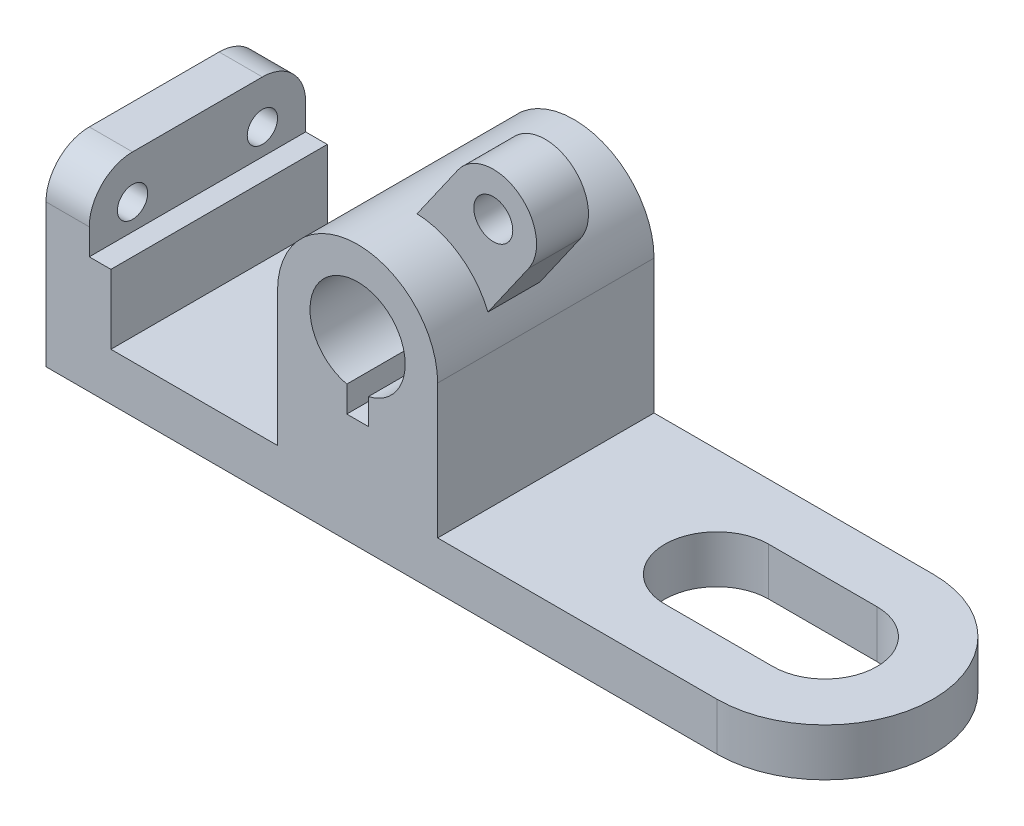
ISO-10303-21;
HEADER;
FILE_DESCRIPTION(('STEP AP214'),'2;1');
FILE_NAME('part.step','',(''),(''),'','','');
FILE_SCHEMA(('AUTOMOTIVE_DESIGN { 1 0 10303 214 1 1 1 1 }'));
ENDSEC;
DATA;
#1=APPLICATION_CONTEXT('core data for automotive mechanical design processes');
#2=APPLICATION_PROTOCOL_DEFINITION('international standard','automotive_design',2000,#1);
#3=PRODUCT_CONTEXT('',#1,'mechanical');
#4=PRODUCT('Part','Part','',(#3));
#5=PRODUCT_RELATED_PRODUCT_CATEGORY('part','',(#4));
#6=PRODUCT_DEFINITION_FORMATION('','',#4);
#7=PRODUCT_DEFINITION_CONTEXT('part definition',#1,'design');
#8=PRODUCT_DEFINITION('design','',#6,#7);
#9=PRODUCT_DEFINITION_SHAPE('','',#8);
#10=(LENGTH_UNIT() NAMED_UNIT(*) SI_UNIT(.MILLI.,.METRE.));
#11=(NAMED_UNIT(*) PLANE_ANGLE_UNIT() SI_UNIT($,.RADIAN.));
#12=(NAMED_UNIT(*) SI_UNIT($,.STERADIAN.) SOLID_ANGLE_UNIT());
#13=UNCERTAINTY_MEASURE_WITH_UNIT(LENGTH_MEASURE(1.E-05),#10,'distance_accuracy_value','');
#14=(GEOMETRIC_REPRESENTATION_CONTEXT(3) GLOBAL_UNCERTAINTY_ASSIGNED_CONTEXT((#13)) GLOBAL_UNIT_ASSIGNED_CONTEXT((#10,
#11,#12)) REPRESENTATION_CONTEXT('',''));
#15=CARTESIAN_POINT('',(0.,0.,0.));
#16=DIRECTION('',(0.,0.,1.));
#17=DIRECTION('',(1.,0.,0.));
#18=AXIS2_PLACEMENT_3D('',#15,#16,#17);
#19=CARTESIAN_POINT('',(-83.,42.,-25.));
#20=DIRECTION('',(0.,0.,1.));
#21=DIRECTION('',(1.,0.,0.));
#22=AXIS2_PLACEMENT_3D('',#19,#20,#21);
#23=CYLINDRICAL_SURFACE('',#22,18.5);
#24=CARTESIAN_POINT('',(-83.,42.,25.));
#25=DIRECTION('',(0.,0.,1.));
#26=DIRECTION('',(1.,0.,0.));
#27=AXIS2_PLACEMENT_3D('',#24,#25,#26);
#28=CIRCLE('',#27,18.5);
#29=CARTESIAN_POINT('',(-64.5,42.,25.));
#30=VERTEX_POINT('',#29);
#31=CARTESIAN_POINT('',(-101.5,42.,25.));
#32=VERTEX_POINT('',#31);
#33=EDGE_CURVE('E272',#30,#32,#28,.T.);
#34=ORIENTED_EDGE('',*,*,#33,.F.);
#35=DIRECTION('',(0.,0.,1.));
#36=VECTOR('',#35,1.);
#37=CARTESIAN_POINT('',(-64.5,42.,-25.));
#38=LINE('',#37,#36);
#39=CARTESIAN_POINT('',(-64.5,42.,-25.));
#40=VERTEX_POINT('',#39);
#41=EDGE_CURVE('E303',#40,#30,#38,.T.);
#42=ORIENTED_EDGE('',*,*,#41,.F.);
#43=CARTESIAN_POINT('',(-83.,42.,-25.));
#44=DIRECTION('',(0.,0.,1.));
#45=DIRECTION('',(1.,0.,0.));
#46=AXIS2_PLACEMENT_3D('',#43,#44,#45);
#47=CIRCLE('',#46,18.5);
#48=CARTESIAN_POINT('',(-101.5,42.,-25.));
#49=VERTEX_POINT('',#48);
#50=EDGE_CURVE('E255',#40,#49,#47,.T.);
#51=ORIENTED_EDGE('',*,*,#50,.T.);
#52=DIRECTION('',(0.,0.,1.));
#53=VECTOR('',#52,1.);
#54=CARTESIAN_POINT('',(-101.5,42.,-25.));
#55=LINE('',#54,#53);
#56=EDGE_CURVE('E301',#49,#32,#55,.T.);
#57=ORIENTED_EDGE('',*,*,#56,.T.);
#58=EDGE_LOOP('',(#34,#42,#51,#57));
#59=FACE_BOUND('',#58,.T.);
#60=CARTESIAN_POINT('',(-83.,42.,12.));
#61=DIRECTION('',(0.,0.,-1.));
#62=DIRECTION('',(1.,0.,0.));
#63=AXIS2_PLACEMENT_3D('',#60,#61,#62);
#64=CIRCLE('',#63,18.5);
#65=CARTESIAN_POINT('',(-82.264157442559,60.4853600378964,12.));
#66=VERTEX_POINT('',#65);
#67=CARTESIAN_POINT('',(-65.8811165567791,49.0138313108756,12.));
#68=VERTEX_POINT('',#67);
#69=EDGE_CURVE('E227',#66,#68,#64,.T.);
#70=ORIENTED_EDGE('',*,*,#69,.F.);
#71=DIRECTION('',(0.,0.,-1.));
#72=VECTOR('',#71,1.);
#73=CARTESIAN_POINT('',(-82.264157442559,60.4853600378964,12.));
#74=LINE('',#73,#72);
#75=CARTESIAN_POINT('',(-82.264157442559,60.4853600378964,0.));
#76=VERTEX_POINT('',#75);
#77=EDGE_CURVE('E224',#66,#76,#74,.T.);
#78=ORIENTED_EDGE('',*,*,#77,.T.);
#79=CARTESIAN_POINT('',(-83.,42.,0.));
#80=DIRECTION('',(0.,0.,-1.));
#81=DIRECTION('',(1.,0.,0.));
#82=AXIS2_PLACEMENT_3D('',#79,#80,#81);
#83=CIRCLE('',#82,18.5);
#84=CARTESIAN_POINT('',(-65.8811165567791,49.0138313108756,0.));
#85=VERTEX_POINT('',#84);
#86=EDGE_CURVE('E429',#76,#85,#83,.T.);
#87=ORIENTED_EDGE('',*,*,#86,.T.);
#88=DIRECTION('',(0.,0.,-1.));
#89=VECTOR('',#88,1.);
#90=CARTESIAN_POINT('',(-65.8811165567791,49.0138313108756,12.));
#91=LINE('',#90,#89);
#92=EDGE_CURVE('E246',#68,#85,#91,.T.);
#93=ORIENTED_EDGE('',*,*,#92,.F.);
#94=EDGE_LOOP('',(#70,#78,#87,#93));
#95=FACE_BOUND('',#94,.T.);
#96=ADVANCED_FACE('F41',(#59,#95),#23,.T.);
#97=CARTESIAN_POINT('',(0.,11.,0.));
#98=DIRECTION('',(0.,1.,0.));
#99=DIRECTION('',(0.,0.,1.));
#100=AXIS2_PLACEMENT_3D('',#97,#98,#99);
#101=PLANE('',#100);
#102=DIRECTION('',(-1.,0.,0.));
#103=VECTOR('',#102,1.);
#104=CARTESIAN_POINT('',(0.,11.,-12.));
#105=LINE('',#104,#103);
#106=CARTESIAN_POINT('',(0.,11.,-12.));
#107=VERTEX_POINT('',#106);
#108=CARTESIAN_POINT('',(-25.,11.,-12.));
#109=VERTEX_POINT('',#108);
#110=EDGE_CURVE('E332',#107,#109,#105,.T.);
#111=ORIENTED_EDGE('',*,*,#110,.F.);
#112=CARTESIAN_POINT('',(0.,11.,0.));
#113=DIRECTION('',(0.,1.,0.));
#114=DIRECTION('',(0.,0.,1.));
#115=AXIS2_PLACEMENT_3D('',#112,#113,#114);
#116=CIRCLE('',#115,12.);
#117=CARTESIAN_POINT('',(0.,11.,12.));
#118=VERTEX_POINT('',#117);
#119=EDGE_CURVE('E328',#118,#107,#116,.T.);
#120=ORIENTED_EDGE('',*,*,#119,.F.);
#121=DIRECTION('',(1.,0.,0.));
#122=VECTOR('',#121,1.);
#123=CARTESIAN_POINT('',(0.,11.,12.));
#124=LINE('',#123,#122);
#125=CARTESIAN_POINT('',(-25.,11.,12.));
#126=VERTEX_POINT('',#125);
#127=EDGE_CURVE('E340',#126,#118,#124,.T.);
#128=ORIENTED_EDGE('',*,*,#127,.F.);
#129=CARTESIAN_POINT('',(-25.,11.,0.));
#130=DIRECTION('',(0.,1.,0.));
#131=DIRECTION('',(0.,0.,1.));
#132=AXIS2_PLACEMENT_3D('',#129,#130,#131);
#133=CIRCLE('',#132,12.);
#134=EDGE_CURVE('E331',#109,#126,#133,.T.);
#135=ORIENTED_EDGE('',*,*,#134,.F.);
#136=EDGE_LOOP('',(#111,#120,#128,#135));
#137=FACE_BOUND('',#136,.T.);
#138=DIRECTION('',(-1.,0.,0.));
#139=VECTOR('',#138,1.);
#140=CARTESIAN_POINT('',(0.,11.,-25.));
#141=LINE('',#140,#139);
#142=CARTESIAN_POINT('',(0.,11.,-25.));
#143=VERTEX_POINT('',#142);
#144=CARTESIAN_POINT('',(-64.5,11.,-25.));
#145=VERTEX_POINT('',#144);
#146=EDGE_CURVE('E362',#143,#145,#141,.T.);
#147=ORIENTED_EDGE('',*,*,#146,.T.);
#148=DIRECTION('',(0.,0.,1.));
#149=VECTOR('',#148,1.);
#150=CARTESIAN_POINT('',(-64.5,11.,-25.));
#151=LINE('',#150,#149);
#152=CARTESIAN_POINT('',(-64.5,11.,25.));
#153=VERTEX_POINT('',#152);
#154=EDGE_CURVE('E269',#145,#153,#151,.T.);
#155=ORIENTED_EDGE('',*,*,#154,.T.);
#156=DIRECTION('',(1.,0.,0.));
#157=VECTOR('',#156,1.);
#158=CARTESIAN_POINT('',(0.,11.,25.));
#159=LINE('',#158,#157);
#160=CARTESIAN_POINT('',(0.,11.,25.));
#161=VERTEX_POINT('',#160);
#162=EDGE_CURVE('E368',#153,#161,#159,.T.);
#163=ORIENTED_EDGE('',*,*,#162,.T.);
#164=CARTESIAN_POINT('',(0.,11.,0.));
#165=DIRECTION('',(0.,1.,0.));
#166=DIRECTION('',(0.,0.,1.));
#167=AXIS2_PLACEMENT_3D('',#164,#165,#166);
#168=CIRCLE('',#167,25.);
#169=EDGE_CURVE('E359',#161,#143,#168,.T.);
#170=ORIENTED_EDGE('',*,*,#169,.T.);
#171=EDGE_LOOP('',(#147,#155,#163,#170));
#172=FACE_BOUND('',#171,.T.);
#173=ADVANCED_FACE('F442',(#137,#172),#101,.T.);
#174=DIRECTION('',(0.,0.,1.));
#175=VECTOR('',#174,1.);
#176=CARTESIAN_POINT('',(-101.5,11.,-25.));
#177=LINE('',#176,#175);
#178=CARTESIAN_POINT('',(-101.5,11.,-25.));
#179=VERTEX_POINT('',#178);
#180=CARTESIAN_POINT('',(-101.5,11.,25.));
#181=VERTEX_POINT('',#180);
#182=EDGE_CURVE('E299',#179,#181,#177,.T.);
#183=ORIENTED_EDGE('',*,*,#182,.F.);
#184=CARTESIAN_POINT('',(-140.,11.,-25.));
#185=VERTEX_POINT('',#184);
#186=EDGE_CURVE('E361',#179,#185,#141,.T.);
#187=ORIENTED_EDGE('',*,*,#186,.T.);
#188=DIRECTION('',(0.,0.,1.));
#189=VECTOR('',#188,1.);
#190=CARTESIAN_POINT('',(-140.,11.,-25.));
#191=LINE('',#190,#189);
#192=CARTESIAN_POINT('',(-140.,11.,25.));
#193=VERTEX_POINT('',#192);
#194=EDGE_CURVE('E275',#185,#193,#191,.T.);
#195=ORIENTED_EDGE('',*,*,#194,.T.);
#196=EDGE_CURVE('E369',#193,#181,#159,.T.);
#197=ORIENTED_EDGE('',*,*,#196,.T.);
#198=EDGE_LOOP('',(#183,#187,#195,#197));
#199=FACE_BOUND('',#198,.T.);
#200=ADVANCED_FACE('F452',(#199),#101,.T.);
#201=CARTESIAN_POINT('',(0.,0.,0.));
#202=DIRECTION('',(0.,1.,0.));
#203=DIRECTION('',(0.,0.,1.));
#204=AXIS2_PLACEMENT_3D('',#201,#202,#203);
#205=PLANE('',#204);
#206=CARTESIAN_POINT('',(0.,0.,0.));
#207=DIRECTION('',(0.,1.,0.));
#208=DIRECTION('',(0.,0.,1.));
#209=AXIS2_PLACEMENT_3D('',#206,#207,#208);
#210=CIRCLE('',#209,25.);
#211=CARTESIAN_POINT('',(0.,0.,25.));
#212=VERTEX_POINT('',#211);
#213=CARTESIAN_POINT('',(0.,0.,-25.));
#214=VERTEX_POINT('',#213);
#215=EDGE_CURVE('E360',#212,#214,#210,.T.);
#216=ORIENTED_EDGE('',*,*,#215,.F.);
#217=DIRECTION('',(1.,0.,0.));
#218=VECTOR('',#217,1.);
#219=CARTESIAN_POINT('',(0.,0.,25.));
#220=LINE('',#219,#218);
#221=CARTESIAN_POINT('',(-155.,0.,25.));
#222=VERTEX_POINT('',#221);
#223=EDGE_CURVE('E364',#222,#212,#220,.T.);
#224=ORIENTED_EDGE('',*,*,#223,.F.);
#225=DIRECTION('',(0.,0.,1.));
#226=VECTOR('',#225,1.);
#227=CARTESIAN_POINT('',(-155.,0.,25.));
#228=LINE('',#227,#226);
#229=CARTESIAN_POINT('',(-155.,0.,-25.));
#230=VERTEX_POINT('',#229);
#231=EDGE_CURVE('E376',#230,#222,#228,.T.);
#232=ORIENTED_EDGE('',*,*,#231,.F.);
#233=DIRECTION('',(-1.,0.,0.));
#234=VECTOR('',#233,1.);
#235=CARTESIAN_POINT('',(0.,0.,-25.));
#236=LINE('',#235,#234);
#237=EDGE_CURVE('E373',#214,#230,#236,.T.);
#238=ORIENTED_EDGE('',*,*,#237,.F.);
#239=EDGE_LOOP('',(#216,#224,#232,#238));
#240=FACE_BOUND('',#239,.T.);
#241=CARTESIAN_POINT('',(0.,0.,0.));
#242=DIRECTION('',(0.,1.,0.));
#243=DIRECTION('',(0.,0.,1.));
#244=AXIS2_PLACEMENT_3D('',#241,#242,#243);
#245=CIRCLE('',#244,12.);
#246=CARTESIAN_POINT('',(0.,0.,12.));
#247=VERTEX_POINT('',#246);
#248=CARTESIAN_POINT('',(0.,0.,-12.));
#249=VERTEX_POINT('',#248);
#250=EDGE_CURVE('E293',#247,#249,#245,.T.);
#251=ORIENTED_EDGE('',*,*,#250,.T.);
#252=DIRECTION('',(-1.,0.,0.));
#253=VECTOR('',#252,1.);
#254=CARTESIAN_POINT('',(0.,0.,-12.));
#255=LINE('',#254,#253);
#256=CARTESIAN_POINT('',(-25.,0.,-12.));
#257=VERTEX_POINT('',#256);
#258=EDGE_CURVE('E345',#249,#257,#255,.T.);
#259=ORIENTED_EDGE('',*,*,#258,.T.);
#260=CARTESIAN_POINT('',(-25.,0.,0.));
#261=DIRECTION('',(0.,1.,0.));
#262=DIRECTION('',(0.,0.,1.));
#263=AXIS2_PLACEMENT_3D('',#260,#261,#262);
#264=CIRCLE('',#263,12.);
#265=CARTESIAN_POINT('',(-25.,0.,12.));
#266=VERTEX_POINT('',#265);
#267=EDGE_CURVE('E343',#257,#266,#264,.T.);
#268=ORIENTED_EDGE('',*,*,#267,.T.);
#269=DIRECTION('',(1.,0.,0.));
#270=VECTOR('',#269,1.);
#271=CARTESIAN_POINT('',(0.,0.,12.));
#272=LINE('',#271,#270);
#273=EDGE_CURVE('E335',#266,#247,#272,.T.);
#274=ORIENTED_EDGE('',*,*,#273,.T.);
#275=EDGE_LOOP('',(#251,#259,#268,#274));
#276=FACE_BOUND('',#275,.T.);
#277=ADVANCED_FACE('F498',(#240,#276),#205,.F.);
#278=CARTESIAN_POINT('',(0.,11.,0.));
#279=DIRECTION('',(0.,-1.,0.));
#280=DIRECTION('',(0.,0.,-1.));
#281=AXIS2_PLACEMENT_3D('',#278,#279,#280);
#282=CYLINDRICAL_SURFACE('',#281,25.);
#283=ORIENTED_EDGE('',*,*,#215,.T.);
#284=DIRECTION('',(0.,-1.,0.));
#285=VECTOR('',#284,1.);
#286=CARTESIAN_POINT('',(0.,11.,-25.));
#287=LINE('',#286,#285);
#288=EDGE_CURVE('E390',#143,#214,#287,.T.);
#289=ORIENTED_EDGE('',*,*,#288,.F.);
#290=ORIENTED_EDGE('',*,*,#169,.F.);
#291=DIRECTION('',(0.,-1.,0.));
#292=VECTOR('',#291,1.);
#293=CARTESIAN_POINT('',(0.,11.,25.));
#294=LINE('',#293,#292);
#295=EDGE_CURVE('E379',#161,#212,#294,.T.);
#296=ORIENTED_EDGE('',*,*,#295,.T.);
#297=EDGE_LOOP('',(#283,#289,#290,#296));
#298=FACE_BOUND('',#297,.T.);
#299=ADVANCED_FACE('F501',(#298),#282,.T.);
#300=CARTESIAN_POINT('',(0.,11.,-25.));
#301=DIRECTION('',(0.,0.,1.));
#302=DIRECTION('',(1.,0.,0.));
#303=AXIS2_PLACEMENT_3D('',#300,#301,#302);
#304=PLANE('',#303);
#305=DIRECTION('',(0.,-1.,0.));
#306=VECTOR('',#305,1.);
#307=CARTESIAN_POINT('',(-155.,11.,-25.));
#308=LINE('',#307,#306);
#309=CARTESIAN_POINT('',(-155.,33.,-25.));
#310=VERTEX_POINT('',#309);
#311=EDGE_CURVE('E383',#310,#230,#308,.T.);
#312=ORIENTED_EDGE('',*,*,#311,.F.);
#313=DIRECTION('',(1.,0.,0.));
#314=VECTOR('',#313,1.);
#315=CARTESIAN_POINT('',(0.,33.,-25.));
#316=LINE('',#315,#314);
#317=CARTESIAN_POINT('',(-145.,33.,-25.));
#318=VERTEX_POINT('',#317);
#319=EDGE_CURVE('E388',#310,#318,#316,.T.);
#320=ORIENTED_EDGE('',*,*,#319,.T.);
#321=DIRECTION('',(0.,-1.,0.));
#322=VECTOR('',#321,1.);
#323=CARTESIAN_POINT('',(-145.,-2.51534904016637E-13,-25.));
#324=LINE('',#323,#322);
#325=CARTESIAN_POINT('',(-145.,27.,-25.));
#326=VERTEX_POINT('',#325);
#327=EDGE_CURVE('E315',#318,#326,#324,.T.);
#328=ORIENTED_EDGE('',*,*,#327,.T.);
#329=DIRECTION('',(1.,0.,0.));
#330=VECTOR('',#329,1.);
#331=CARTESIAN_POINT('',(0.,27.,-25.));
#332=LINE('',#331,#330);
#333=CARTESIAN_POINT('',(-140.,27.,-25.));
#334=VERTEX_POINT('',#333);
#335=EDGE_CURVE('E307',#326,#334,#332,.T.);
#336=ORIENTED_EDGE('',*,*,#335,.T.);
#337=DIRECTION('',(0.,-1.,0.));
#338=VECTOR('',#337,1.);
#339=CARTESIAN_POINT('',(-140.,0.,-25.));
#340=LINE('',#339,#338);
#341=EDGE_CURVE('E310',#334,#185,#340,.T.);
#342=ORIENTED_EDGE('',*,*,#341,.T.);
#343=ORIENTED_EDGE('',*,*,#186,.F.);
#344=DIRECTION('',(0.,-1.,0.));
#345=VECTOR('',#344,1.);
#346=CARTESIAN_POINT('',(-101.5,0.,-25.));
#347=LINE('',#346,#345);
#348=EDGE_CURVE('E257',#49,#179,#347,.T.);
#349=ORIENTED_EDGE('',*,*,#348,.F.);
#350=ORIENTED_EDGE('',*,*,#50,.F.);
#351=DIRECTION('',(0.,-1.,0.));
#352=VECTOR('',#351,1.);
#353=CARTESIAN_POINT('',(-64.5,0.,-25.));
#354=LINE('',#353,#352);
#355=EDGE_CURVE('E249',#40,#145,#354,.T.);
#356=ORIENTED_EDGE('',*,*,#355,.T.);
#357=ORIENTED_EDGE('',*,*,#146,.F.);
#358=ORIENTED_EDGE('',*,*,#288,.T.);
#359=ORIENTED_EDGE('',*,*,#237,.T.);
#360=EDGE_LOOP('',(#312,#320,#328,#336,#342,#343,#349,#350,#356,#357,#358,#359));
#361=FACE_BOUND('',#360,.T.);
#362=DIRECTION('',(0.,1.,0.));
#363=VECTOR('',#362,1.);
#364=CARTESIAN_POINT('',(-80.5,0.,-25.));
#365=LINE('',#364,#363);
#366=CARTESIAN_POINT('',(-80.5,25.2878573571857,-25.));
#367=VERTEX_POINT('',#366);
#368=CARTESIAN_POINT('',(-80.5,31.2878573571857,-25.));
#369=VERTEX_POINT('',#368);
#370=EDGE_CURVE('E259',#367,#369,#365,.T.);
#371=ORIENTED_EDGE('',*,*,#370,.T.);
#372=CARTESIAN_POINT('',(-83.,42.,-25.));
#373=DIRECTION('',(0.,0.,1.));
#374=DIRECTION('',(1.,0.,0.));
#375=AXIS2_PLACEMENT_3D('',#372,#373,#374);
#376=CIRCLE('',#375,11.);
#377=CARTESIAN_POINT('',(-85.5,31.2878573571857,-25.));
#378=VERTEX_POINT('',#377);
#379=EDGE_CURVE('E267',#369,#378,#376,.T.);
#380=ORIENTED_EDGE('',*,*,#379,.T.);
#381=DIRECTION('',(0.,1.,0.));
#382=VECTOR('',#381,1.);
#383=CARTESIAN_POINT('',(-85.5,0.,-25.));
#384=LINE('',#383,#382);
#385=CARTESIAN_POINT('',(-85.5,25.2878573571857,-25.));
#386=VERTEX_POINT('',#385);
#387=EDGE_CURVE('E262',#386,#378,#384,.T.);
#388=ORIENTED_EDGE('',*,*,#387,.F.);
#389=DIRECTION('',(1.,0.,0.));
#390=VECTOR('',#389,1.);
#391=CARTESIAN_POINT('',(0.,25.2878573571857,-25.));
#392=LINE('',#391,#390);
#393=EDGE_CURVE('E261',#386,#367,#392,.T.);
#394=ORIENTED_EDGE('',*,*,#393,.T.);
#395=EDGE_LOOP('',(#371,#380,#388,#394));
#396=FACE_BOUND('',#395,.T.);
#397=ADVANCED_FACE('F507',(#361,#396),#304,.F.);
#398=CARTESIAN_POINT('',(-155.,11.,25.));
#399=DIRECTION('',(1.,0.,0.));
#400=DIRECTION('',(0.,0.,-1.));
#401=AXIS2_PLACEMENT_3D('',#398,#399,#400);
#402=PLANE('',#401);
#403=CARTESIAN_POINT('',(-155.,33.,15.));
#404=DIRECTION('',(-1.,0.,0.));
#405=DIRECTION('',(0.,0.,1.));
#406=AXIS2_PLACEMENT_3D('',#403,#404,#405);
#407=CIRCLE('',#406,3.5);
#408=CARTESIAN_POINT('',(-155.,33.,18.5));
#409=VERTEX_POINT('',#408);
#410=EDGE_CURVE('E403',#409,#409,#407,.T.);
#411=ORIENTED_EDGE('',*,*,#410,.F.);
#412=EDGE_LOOP('',(#411));
#413=FACE_BOUND('',#412,.T.);
#414=CARTESIAN_POINT('',(-155.,33.,-15.));
#415=DIRECTION('',(-1.,0.,0.));
#416=DIRECTION('',(0.,0.,1.));
#417=AXIS2_PLACEMENT_3D('',#414,#415,#416);
#418=CIRCLE('',#417,3.5);
#419=CARTESIAN_POINT('',(-155.,33.,-11.5));
#420=VERTEX_POINT('',#419);
#421=EDGE_CURVE('E411',#420,#420,#418,.T.);
#422=ORIENTED_EDGE('',*,*,#421,.F.);
#423=EDGE_LOOP('',(#422));
#424=FACE_BOUND('',#423,.T.);
#425=DIRECTION('',(0.,0.,1.));
#426=VECTOR('',#425,1.);
#427=CARTESIAN_POINT('',(-155.,43.,-25.));
#428=LINE('',#427,#426);
#429=CARTESIAN_POINT('',(-155.,43.,-15.));
#430=VERTEX_POINT('',#429);
#431=CARTESIAN_POINT('',(-155.,43.,15.));
#432=VERTEX_POINT('',#431);
#433=EDGE_CURVE('E316',#430,#432,#428,.T.);
#434=ORIENTED_EDGE('',*,*,#433,.F.);
#435=CARTESIAN_POINT('',(-155.,33.,-15.));
#436=DIRECTION('',(1.,0.,0.));
#437=DIRECTION('',(0.,0.,-1.));
#438=AXIS2_PLACEMENT_3D('',#435,#436,#437);
#439=CIRCLE('',#438,10.);
#440=EDGE_CURVE('E49',#430,#310,#439,.F.);
#441=ORIENTED_EDGE('',*,*,#440,.T.);
#442=ORIENTED_EDGE('',*,*,#311,.T.);
#443=ORIENTED_EDGE('',*,*,#231,.T.);
#444=DIRECTION('',(0.,-1.,0.));
#445=VECTOR('',#444,1.);
#446=CARTESIAN_POINT('',(-155.,11.,25.));
#447=LINE('',#446,#445);
#448=CARTESIAN_POINT('',(-155.,33.,25.));
#449=VERTEX_POINT('',#448);
#450=EDGE_CURVE('E384',#449,#222,#447,.T.);
#451=ORIENTED_EDGE('',*,*,#450,.F.);
#452=CARTESIAN_POINT('',(-155.,33.,15.));
#453=DIRECTION('',(1.,0.,0.));
#454=DIRECTION('',(0.,0.,-1.));
#455=AXIS2_PLACEMENT_3D('',#452,#453,#454);
#456=CIRCLE('',#455,10.);
#457=EDGE_CURVE('E64',#449,#432,#456,.F.);
#458=ORIENTED_EDGE('',*,*,#457,.T.);
#459=EDGE_LOOP('',(#434,#441,#442,#443,#451,#458));
#460=FACE_BOUND('',#459,.T.);
#461=ADVANCED_FACE('F504',(#413,#424,#460),#402,.F.);
#462=CARTESIAN_POINT('',(0.,11.,25.));
#463=DIRECTION('',(0.,0.,-1.));
#464=DIRECTION('',(-1.,0.,0.));
#465=AXIS2_PLACEMENT_3D('',#462,#463,#464);
#466=PLANE('',#465);
#467=DIRECTION('',(0.,-1.,0.));
#468=VECTOR('',#467,1.);
#469=CARTESIAN_POINT('',(-145.,-2.51534904016637E-13,25.));
#470=LINE('',#469,#468);
#471=CARTESIAN_POINT('',(-145.,33.,25.));
#472=VERTEX_POINT('',#471);
#473=CARTESIAN_POINT('',(-145.,27.,25.));
#474=VERTEX_POINT('',#473);
#475=EDGE_CURVE('E309',#472,#474,#470,.T.);
#476=ORIENTED_EDGE('',*,*,#475,.F.);
#477=DIRECTION('',(1.,0.,0.));
#478=VECTOR('',#477,1.);
#479=CARTESIAN_POINT('',(0.,33.,25.));
#480=LINE('',#479,#478);
#481=EDGE_CURVE('E11',#472,#449,#480,.F.);
#482=ORIENTED_EDGE('',*,*,#481,.T.);
#483=ORIENTED_EDGE('',*,*,#450,.T.);
#484=ORIENTED_EDGE('',*,*,#223,.T.);
#485=ORIENTED_EDGE('',*,*,#295,.F.);
#486=ORIENTED_EDGE('',*,*,#162,.F.);
#487=DIRECTION('',(0.,-1.,0.));
#488=VECTOR('',#487,1.);
#489=CARTESIAN_POINT('',(-64.5,0.,25.));
#490=LINE('',#489,#488);
#491=EDGE_CURVE('E266',#30,#153,#490,.T.);
#492=ORIENTED_EDGE('',*,*,#491,.F.);
#493=ORIENTED_EDGE('',*,*,#33,.T.);
#494=DIRECTION('',(0.,-1.,0.));
#495=VECTOR('',#494,1.);
#496=CARTESIAN_POINT('',(-101.5,0.,25.));
#497=LINE('',#496,#495);
#498=EDGE_CURVE('E273',#32,#181,#497,.T.);
#499=ORIENTED_EDGE('',*,*,#498,.T.);
#500=ORIENTED_EDGE('',*,*,#196,.F.);
#501=DIRECTION('',(0.,-1.,0.));
#502=VECTOR('',#501,1.);
#503=CARTESIAN_POINT('',(-140.,0.,25.));
#504=LINE('',#503,#502);
#505=CARTESIAN_POINT('',(-140.,27.,25.));
#506=VERTEX_POINT('',#505);
#507=EDGE_CURVE('E245',#506,#193,#504,.T.);
#508=ORIENTED_EDGE('',*,*,#507,.F.);
#509=DIRECTION('',(1.,0.,0.));
#510=VECTOR('',#509,1.);
#511=CARTESIAN_POINT('',(0.,27.,25.));
#512=LINE('',#511,#510);
#513=EDGE_CURVE('E242',#474,#506,#512,.T.);
#514=ORIENTED_EDGE('',*,*,#513,.F.);
#515=EDGE_LOOP('',(#476,#482,#483,#484,#485,#486,#492,#493,#499,#500,#508,#514));
#516=FACE_BOUND('',#515,.T.);
#517=DIRECTION('',(0.,1.,0.));
#518=VECTOR('',#517,1.);
#519=CARTESIAN_POINT('',(-80.5,0.,25.));
#520=LINE('',#519,#518);
#521=CARTESIAN_POINT('',(-80.5,25.2878573571857,25.));
#522=VERTEX_POINT('',#521);
#523=CARTESIAN_POINT('',(-80.5,31.2878573571857,25.));
#524=VERTEX_POINT('',#523);
#525=EDGE_CURVE('E279',#522,#524,#520,.T.);
#526=ORIENTED_EDGE('',*,*,#525,.F.);
#527=DIRECTION('',(1.,0.,0.));
#528=VECTOR('',#527,1.);
#529=CARTESIAN_POINT('',(0.,25.2878573571857,25.));
#530=LINE('',#529,#528);
#531=CARTESIAN_POINT('',(-85.5,25.2878573571857,25.));
#532=VERTEX_POINT('',#531);
#533=EDGE_CURVE('E281',#532,#522,#530,.T.);
#534=ORIENTED_EDGE('',*,*,#533,.F.);
#535=DIRECTION('',(0.,1.,0.));
#536=VECTOR('',#535,1.);
#537=CARTESIAN_POINT('',(-85.5,0.,25.));
#538=LINE('',#537,#536);
#539=CARTESIAN_POINT('',(-85.5,31.2878573571857,25.));
#540=VERTEX_POINT('',#539);
#541=EDGE_CURVE('E282',#532,#540,#538,.T.);
#542=ORIENTED_EDGE('',*,*,#541,.T.);
#543=CARTESIAN_POINT('',(-83.,42.,25.));
#544=DIRECTION('',(0.,0.,1.));
#545=DIRECTION('',(1.,0.,0.));
#546=AXIS2_PLACEMENT_3D('',#543,#544,#545);
#547=CIRCLE('',#546,11.);
#548=EDGE_CURVE('E254',#524,#540,#547,.T.);
#549=ORIENTED_EDGE('',*,*,#548,.F.);
#550=EDGE_LOOP('',(#526,#534,#542,#549));
#551=FACE_BOUND('',#550,.T.);
#552=ADVANCED_FACE('F492',(#516,#551),#466,.F.);
#553=CARTESIAN_POINT('',(0.,11.,0.));
#554=DIRECTION('',(0.,-1.,0.));
#555=DIRECTION('',(0.,0.,-1.));
#556=AXIS2_PLACEMENT_3D('',#553,#554,#555);
#557=CYLINDRICAL_SURFACE('',#556,12.);
#558=ORIENTED_EDGE('',*,*,#250,.F.);
#559=DIRECTION('',(0.,-1.,0.));
#560=VECTOR('',#559,1.);
#561=CARTESIAN_POINT('',(0.,11.,12.));
#562=LINE('',#561,#560);
#563=EDGE_CURVE('E339',#118,#247,#562,.T.);
#564=ORIENTED_EDGE('',*,*,#563,.F.);
#565=ORIENTED_EDGE('',*,*,#119,.T.);
#566=DIRECTION('',(0.,-1.,0.));
#567=VECTOR('',#566,1.);
#568=CARTESIAN_POINT('',(0.,11.,-12.));
#569=LINE('',#568,#567);
#570=EDGE_CURVE('E358',#107,#249,#569,.T.);
#571=ORIENTED_EDGE('',*,*,#570,.T.);
#572=EDGE_LOOP('',(#558,#564,#565,#571));
#573=FACE_BOUND('',#572,.T.);
#574=ADVANCED_FACE('F495',(#573),#557,.F.);
#575=CARTESIAN_POINT('',(0.,11.,-12.));
#576=DIRECTION('',(0.,0.,1.));
#577=DIRECTION('',(1.,0.,0.));
#578=AXIS2_PLACEMENT_3D('',#575,#576,#577);
#579=PLANE('',#578);
#580=ORIENTED_EDGE('',*,*,#258,.F.);
#581=ORIENTED_EDGE('',*,*,#570,.F.);
#582=ORIENTED_EDGE('',*,*,#110,.T.);
#583=DIRECTION('',(0.,-1.,0.));
#584=VECTOR('',#583,1.);
#585=CARTESIAN_POINT('',(-25.,11.,-12.));
#586=LINE('',#585,#584);
#587=EDGE_CURVE('E351',#109,#257,#586,.T.);
#588=ORIENTED_EDGE('',*,*,#587,.T.);
#589=EDGE_LOOP('',(#580,#581,#582,#588));
#590=FACE_BOUND('',#589,.T.);
#591=ADVANCED_FACE('F486',(#590),#579,.T.);
#592=CARTESIAN_POINT('',(-25.,11.,0.));
#593=DIRECTION('',(0.,-1.,0.));
#594=DIRECTION('',(0.,0.,-1.));
#595=AXIS2_PLACEMENT_3D('',#592,#593,#594);
#596=CYLINDRICAL_SURFACE('',#595,12.);
#597=ORIENTED_EDGE('',*,*,#267,.F.);
#598=ORIENTED_EDGE('',*,*,#587,.F.);
#599=ORIENTED_EDGE('',*,*,#134,.T.);
#600=DIRECTION('',(0.,-1.,0.));
#601=VECTOR('',#600,1.);
#602=CARTESIAN_POINT('',(-25.,11.,12.));
#603=LINE('',#602,#601);
#604=EDGE_CURVE('E355',#126,#266,#603,.T.);
#605=ORIENTED_EDGE('',*,*,#604,.T.);
#606=EDGE_LOOP('',(#597,#598,#599,#605));
#607=FACE_BOUND('',#606,.T.);
#608=ADVANCED_FACE('F481',(#607),#596,.F.);
#609=CARTESIAN_POINT('',(0.,11.,12.));
#610=DIRECTION('',(0.,0.,-1.));
#611=DIRECTION('',(-1.,0.,0.));
#612=AXIS2_PLACEMENT_3D('',#609,#610,#611);
#613=PLANE('',#612);
#614=ORIENTED_EDGE('',*,*,#273,.F.);
#615=ORIENTED_EDGE('',*,*,#604,.F.);
#616=ORIENTED_EDGE('',*,*,#127,.T.);
#617=ORIENTED_EDGE('',*,*,#563,.T.);
#618=EDGE_LOOP('',(#614,#615,#616,#617));
#619=FACE_BOUND('',#618,.T.);
#620=ADVANCED_FACE('F479',(#619),#613,.T.);
#621=CARTESIAN_POINT('',(-140.,0.,-25.));
#622=DIRECTION('',(-1.,0.,0.));
#623=DIRECTION('',(0.,0.,1.));
#624=AXIS2_PLACEMENT_3D('',#621,#622,#623);
#625=PLANE('',#624);
#626=ORIENTED_EDGE('',*,*,#507,.T.);
#627=ORIENTED_EDGE('',*,*,#194,.F.);
#628=ORIENTED_EDGE('',*,*,#341,.F.);
#629=DIRECTION('',(0.,0.,1.));
#630=VECTOR('',#629,1.);
#631=CARTESIAN_POINT('',(-140.,27.,-25.));
#632=LINE('',#631,#630);
#633=EDGE_CURVE('E312',#334,#506,#632,.T.);
#634=ORIENTED_EDGE('',*,*,#633,.T.);
#635=EDGE_LOOP('',(#626,#627,#628,#634));
#636=FACE_BOUND('',#635,.T.);
#637=ADVANCED_FACE('F466',(#636),#625,.F.);
#638=CARTESIAN_POINT('',(0.,43.,-25.));
#639=DIRECTION('',(0.,-1.,0.));
#640=DIRECTION('',(0.,0.,-1.));
#641=AXIS2_PLACEMENT_3D('',#638,#639,#640);
#642=PLANE('',#641);
#643=DIRECTION('',(0.,0.,1.));
#644=VECTOR('',#643,1.);
#645=CARTESIAN_POINT('',(-145.,43.,-25.));
#646=LINE('',#645,#644);
#647=CARTESIAN_POINT('',(-145.,43.,-15.));
#648=VERTEX_POINT('',#647);
#649=CARTESIAN_POINT('',(-145.,43.,15.));
#650=VERTEX_POINT('',#649);
#651=EDGE_CURVE('E322',#648,#650,#646,.T.);
#652=ORIENTED_EDGE('',*,*,#651,.F.);
#653=DIRECTION('',(1.,0.,0.));
#654=VECTOR('',#653,1.);
#655=CARTESIAN_POINT('',(0.,43.,-15.));
#656=LINE('',#655,#654);
#657=EDGE_CURVE('E398',#648,#430,#656,.F.);
#658=ORIENTED_EDGE('',*,*,#657,.T.);
#659=ORIENTED_EDGE('',*,*,#433,.T.);
#660=DIRECTION('',(1.,0.,0.));
#661=VECTOR('',#660,1.);
#662=CARTESIAN_POINT('',(0.,43.,15.));
#663=LINE('',#662,#661);
#664=EDGE_CURVE('E400',#432,#650,#663,.T.);
#665=ORIENTED_EDGE('',*,*,#664,.T.);
#666=EDGE_LOOP('',(#652,#658,#659,#665));
#667=FACE_BOUND('',#666,.T.);
#668=ADVANCED_FACE('F461',(#667),#642,.F.);
#669=CARTESIAN_POINT('',(-145.,-2.51534904016637E-13,-25.));
#670=DIRECTION('',(-1.,0.,0.));
#671=DIRECTION('',(0.,-1.,0.));
#672=AXIS2_PLACEMENT_3D('',#669,#670,#671);
#673=PLANE('',#672);
#674=CARTESIAN_POINT('',(-145.,33.,15.));
#675=DIRECTION('',(-1.,0.,0.));
#676=DIRECTION('',(0.,-1.,0.));
#677=AXIS2_PLACEMENT_3D('',#674,#675,#676);
#678=CIRCLE('',#677,3.5);
#679=CARTESIAN_POINT('',(-145.,29.5,15.));
#680=VERTEX_POINT('',#679);
#681=EDGE_CURVE('E44',#680,#680,#678,.T.);
#682=ORIENTED_EDGE('',*,*,#681,.T.);
#683=EDGE_LOOP('',(#682));
#684=FACE_BOUND('',#683,.T.);
#685=CARTESIAN_POINT('',(-145.,33.,-15.));
#686=DIRECTION('',(-1.,0.,0.));
#687=DIRECTION('',(0.,-1.,0.));
#688=AXIS2_PLACEMENT_3D('',#685,#686,#687);
#689=CIRCLE('',#688,3.5);
#690=CARTESIAN_POINT('',(-145.,29.5,-15.));
#691=VERTEX_POINT('',#690);
#692=EDGE_CURVE('E401',#691,#691,#689,.T.);
#693=ORIENTED_EDGE('',*,*,#692,.T.);
#694=EDGE_LOOP('',(#693));
#695=FACE_BOUND('',#694,.T.);
#696=ORIENTED_EDGE('',*,*,#327,.F.);
#697=CARTESIAN_POINT('',(-145.,33.,-15.));
#698=DIRECTION('',(-1.,0.,0.));
#699=DIRECTION('',(0.,-1.,0.));
#700=AXIS2_PLACEMENT_3D('',#697,#698,#699);
#701=CIRCLE('',#700,10.);
#702=EDGE_CURVE('E394',#318,#648,#701,.F.);
#703=ORIENTED_EDGE('',*,*,#702,.T.);
#704=ORIENTED_EDGE('',*,*,#651,.T.);
#705=CARTESIAN_POINT('',(-145.,33.,15.));
#706=DIRECTION('',(-1.,0.,0.));
#707=DIRECTION('',(0.,-1.,0.));
#708=AXIS2_PLACEMENT_3D('',#705,#706,#707);
#709=CIRCLE('',#708,10.);
#710=EDGE_CURVE('E392',#650,#472,#709,.F.);
#711=ORIENTED_EDGE('',*,*,#710,.T.);
#712=ORIENTED_EDGE('',*,*,#475,.T.);
#713=DIRECTION('',(0.,0.,1.));
#714=VECTOR('',#713,1.);
#715=CARTESIAN_POINT('',(-145.,27.,-25.));
#716=LINE('',#715,#714);
#717=EDGE_CURVE('E321',#326,#474,#716,.T.);
#718=ORIENTED_EDGE('',*,*,#717,.F.);
#719=EDGE_LOOP('',(#696,#703,#704,#711,#712,#718));
#720=FACE_BOUND('',#719,.T.);
#721=ADVANCED_FACE('F470',(#684,#695,#720),#673,.F.);
#722=CARTESIAN_POINT('',(0.,27.,-25.));
#723=DIRECTION('',(0.,-1.,0.));
#724=DIRECTION('',(0.,0.,-1.));
#725=AXIS2_PLACEMENT_3D('',#722,#723,#724);
#726=PLANE('',#725);
#727=ORIENTED_EDGE('',*,*,#513,.T.);
#728=ORIENTED_EDGE('',*,*,#633,.F.);
#729=ORIENTED_EDGE('',*,*,#335,.F.);
#730=ORIENTED_EDGE('',*,*,#717,.T.);
#731=EDGE_LOOP('',(#727,#728,#729,#730));
#732=FACE_BOUND('',#731,.T.);
#733=ADVANCED_FACE('F475',(#732),#726,.F.);
#734=CARTESIAN_POINT('',(-80.5,0.,-25.));
#735=DIRECTION('',(1.,0.,0.));
#736=DIRECTION('',(0.,0.,-1.));
#737=AXIS2_PLACEMENT_3D('',#734,#735,#736);
#738=PLANE('',#737);
#739=ORIENTED_EDGE('',*,*,#525,.T.);
#740=DIRECTION('',(0.,0.,1.));
#741=VECTOR('',#740,1.);
#742=CARTESIAN_POINT('',(-80.5,31.2878573571857,-25.));
#743=LINE('',#742,#741);
#744=EDGE_CURVE('E289',#369,#524,#743,.T.);
#745=ORIENTED_EDGE('',*,*,#744,.F.);
#746=ORIENTED_EDGE('',*,*,#370,.F.);
#747=DIRECTION('',(0.,0.,1.));
#748=VECTOR('',#747,1.);
#749=CARTESIAN_POINT('',(-80.5,25.2878573571857,-25.));
#750=LINE('',#749,#748);
#751=EDGE_CURVE('E298',#367,#522,#750,.T.);
#752=ORIENTED_EDGE('',*,*,#751,.T.);
#753=EDGE_LOOP('',(#739,#745,#746,#752));
#754=FACE_BOUND('',#753,.T.);
#755=ADVANCED_FACE('F476',(#754),#738,.F.);
#756=CARTESIAN_POINT('',(-83.,42.,-25.));
#757=DIRECTION('',(0.,0.,1.));
#758=DIRECTION('',(1.,0.,0.));
#759=AXIS2_PLACEMENT_3D('',#756,#757,#758);
#760=CYLINDRICAL_SURFACE('',#759,11.);
#761=ORIENTED_EDGE('',*,*,#548,.T.);
#762=DIRECTION('',(0.,0.,1.));
#763=VECTOR('',#762,1.);
#764=CARTESIAN_POINT('',(-85.5,31.2878573571857,-25.));
#765=LINE('',#764,#763);
#766=EDGE_CURVE('E292',#378,#540,#765,.T.);
#767=ORIENTED_EDGE('',*,*,#766,.F.);
#768=ORIENTED_EDGE('',*,*,#379,.F.);
#769=ORIENTED_EDGE('',*,*,#744,.T.);
#770=EDGE_LOOP('',(#761,#767,#768,#769));
#771=FACE_BOUND('',#770,.T.);
#772=ADVANCED_FACE('F578',(#771),#760,.F.);
#773=CARTESIAN_POINT('',(-85.5,0.,-25.));
#774=DIRECTION('',(1.,0.,0.));
#775=DIRECTION('',(0.,0.,-1.));
#776=AXIS2_PLACEMENT_3D('',#773,#774,#775);
#777=PLANE('',#776);
#778=ORIENTED_EDGE('',*,*,#541,.F.);
#779=DIRECTION('',(0.,0.,1.));
#780=VECTOR('',#779,1.);
#781=CARTESIAN_POINT('',(-85.5,25.2878573571857,-25.));
#782=LINE('',#781,#780);
#783=EDGE_CURVE('E295',#386,#532,#782,.T.);
#784=ORIENTED_EDGE('',*,*,#783,.F.);
#785=ORIENTED_EDGE('',*,*,#387,.T.);
#786=ORIENTED_EDGE('',*,*,#766,.T.);
#787=EDGE_LOOP('',(#778,#784,#785,#786));
#788=FACE_BOUND('',#787,.T.);
#789=ADVANCED_FACE('F580',(#788),#777,.T.);
#790=CARTESIAN_POINT('',(-101.5,0.,-25.));
#791=DIRECTION('',(-1.,0.,0.));
#792=DIRECTION('',(0.,0.,1.));
#793=AXIS2_PLACEMENT_3D('',#790,#791,#792);
#794=PLANE('',#793);
#795=ORIENTED_EDGE('',*,*,#498,.F.);
#796=ORIENTED_EDGE('',*,*,#56,.F.);
#797=ORIENTED_EDGE('',*,*,#348,.T.);
#798=ORIENTED_EDGE('',*,*,#182,.T.);
#799=EDGE_LOOP('',(#795,#796,#797,#798));
#800=FACE_BOUND('',#799,.T.);
#801=ADVANCED_FACE('F460',(#800),#794,.T.);
#802=CARTESIAN_POINT('',(-64.5,0.,-25.));
#803=DIRECTION('',(-1.,0.,0.));
#804=DIRECTION('',(0.,0.,1.));
#805=AXIS2_PLACEMENT_3D('',#802,#803,#804);
#806=PLANE('',#805);
#807=ORIENTED_EDGE('',*,*,#491,.T.);
#808=ORIENTED_EDGE('',*,*,#154,.F.);
#809=ORIENTED_EDGE('',*,*,#355,.F.);
#810=ORIENTED_EDGE('',*,*,#41,.T.);
#811=EDGE_LOOP('',(#807,#808,#809,#810));
#812=FACE_BOUND('',#811,.T.);
#813=ADVANCED_FACE('F458',(#812),#806,.F.);
#814=CARTESIAN_POINT('',(0.,25.2878573571857,-25.));
#815=DIRECTION('',(0.,-1.,0.));
#816=DIRECTION('',(0.,0.,-1.));
#817=AXIS2_PLACEMENT_3D('',#814,#815,#816);
#818=PLANE('',#817);
#819=ORIENTED_EDGE('',*,*,#533,.T.);
#820=ORIENTED_EDGE('',*,*,#751,.F.);
#821=ORIENTED_EDGE('',*,*,#393,.F.);
#822=ORIENTED_EDGE('',*,*,#783,.T.);
#823=EDGE_LOOP('',(#819,#820,#821,#822));
#824=FACE_BOUND('',#823,.T.);
#825=ADVANCED_FACE('F465',(#824),#818,.F.);
#826=CARTESIAN_POINT('',(-64.6455540367666,68.2128654172478,12.));
#827=DIRECTION('',(0.,0.,1.));
#828=DIRECTION('',(1.,0.,0.));
#829=AXIS2_PLACEMENT_3D('',#826,#827,#828);
#830=PLANE('',#829);
#831=CARTESIAN_POINT('',(-64.6455540367666,68.2128654172478,12.));
#832=DIRECTION('',(0.,0.,1.));
#833=DIRECTION('',(1.,0.,0.));
#834=AXIS2_PLACEMENT_3D('',#831,#832,#833);
#835=CIRCLE('',#834,9.99999999999999);
#836=CARTESIAN_POINT('',(-56.4540335938767,62.4771010537373,12.));
#837=VERTEX_POINT('',#836);
#838=CARTESIAN_POINT('',(-72.8370744796565,73.9486297807582,12.));
#839=VERTEX_POINT('',#838);
#840=EDGE_CURVE('E226',#837,#839,#835,.T.);
#841=ORIENTED_EDGE('',*,*,#840,.T.);
#842=DIRECTION('',(-0.573576436351044,-0.819152044288993,0.));
#843=VECTOR('',#842,1.);
#844=CARTESIAN_POINT('',(-82.264157442559,60.4853600378964,12.));
#845=LINE('',#844,#843);
#846=EDGE_CURVE('E216',#839,#66,#845,.T.);
#847=ORIENTED_EDGE('',*,*,#846,.T.);
#848=ORIENTED_EDGE('',*,*,#69,.T.);
#849=DIRECTION('',(0.573576436351044,0.819152044288993,0.));
#850=VECTOR('',#849,1.);
#851=CARTESIAN_POINT('',(-65.8811165567791,49.0138313108756,12.));
#852=LINE('',#851,#850);
#853=EDGE_CURVE('E231',#68,#837,#852,.T.);
#854=ORIENTED_EDGE('',*,*,#853,.T.);
#855=EDGE_LOOP('',(#841,#847,#848,#854));
#856=FACE_BOUND('',#855,.T.);
#857=CARTESIAN_POINT('',(-64.6455540367666,68.2128654172478,12.));
#858=DIRECTION('',(0.,0.,1.));
#859=DIRECTION('',(1.,0.,0.));
#860=AXIS2_PLACEMENT_3D('',#857,#858,#859);
#861=CIRCLE('',#860,4.5);
#862=CARTESIAN_POINT('',(-60.1455540367666,68.2128654172478,12.));
#863=VERTEX_POINT('',#862);
#864=EDGE_CURVE('E419',#863,#863,#861,.T.);
#865=ORIENTED_EDGE('',*,*,#864,.F.);
#866=EDGE_LOOP('',(#865));
#867=FACE_BOUND('',#866,.T.);
#868=ADVANCED_FACE('F233',(#856,#867),#830,.T.);
#869=CARTESIAN_POINT('',(-64.6455540367666,68.2128654172478,0.));
#870=DIRECTION('',(0.,0.,1.));
#871=DIRECTION('',(1.,0.,0.));
#872=AXIS2_PLACEMENT_3D('',#869,#870,#871);
#873=PLANE('',#872);
#874=CARTESIAN_POINT('',(-64.6455540367666,68.2128654172478,0.));
#875=DIRECTION('',(0.,0.,1.));
#876=DIRECTION('',(1.,0.,0.));
#877=AXIS2_PLACEMENT_3D('',#874,#875,#876);
#878=CIRCLE('',#877,9.99999999999999);
#879=CARTESIAN_POINT('',(-56.4540335938767,62.4771010537373,0.));
#880=VERTEX_POINT('',#879);
#881=CARTESIAN_POINT('',(-72.8370744796565,73.9486297807582,0.));
#882=VERTEX_POINT('',#881);
#883=EDGE_CURVE('E241',#880,#882,#878,.T.);
#884=ORIENTED_EDGE('',*,*,#883,.F.);
#885=DIRECTION('',(0.573576436351044,0.819152044288993,0.));
#886=VECTOR('',#885,1.);
#887=CARTESIAN_POINT('',(-65.8811165567791,49.0138313108756,0.));
#888=LINE('',#887,#886);
#889=EDGE_CURVE('E240',#85,#880,#888,.T.);
#890=ORIENTED_EDGE('',*,*,#889,.F.);
#891=ORIENTED_EDGE('',*,*,#86,.F.);
#892=DIRECTION('',(-0.573576436351044,-0.819152044288993,0.));
#893=VECTOR('',#892,1.);
#894=CARTESIAN_POINT('',(-82.264157442559,60.4853600378964,0.));
#895=LINE('',#894,#893);
#896=EDGE_CURVE('E430',#882,#76,#895,.T.);
#897=ORIENTED_EDGE('',*,*,#896,.F.);
#898=EDGE_LOOP('',(#884,#890,#891,#897));
#899=FACE_BOUND('',#898,.T.);
#900=CARTESIAN_POINT('',(-64.6455540367666,68.2128654172478,0.));
#901=DIRECTION('',(0.,0.,1.));
#902=DIRECTION('',(1.,0.,0.));
#903=AXIS2_PLACEMENT_3D('',#900,#901,#902);
#904=CIRCLE('',#903,4.5);
#905=CARTESIAN_POINT('',(-60.1455540367666,68.2128654172478,0.));
#906=VERTEX_POINT('',#905);
#907=EDGE_CURVE('E406',#906,#906,#904,.T.);
#908=ORIENTED_EDGE('',*,*,#907,.T.);
#909=EDGE_LOOP('',(#908));
#910=FACE_BOUND('',#909,.T.);
#911=ADVANCED_FACE('F439',(#899,#910),#873,.F.);
#912=CARTESIAN_POINT('',(-64.6455540367666,68.2128654172478,12.));
#913=DIRECTION('',(0.,0.,-1.));
#914=DIRECTION('',(-1.,0.,0.));
#915=AXIS2_PLACEMENT_3D('',#912,#913,#914);
#916=CYLINDRICAL_SURFACE('',#915,9.99999999999999);
#917=ORIENTED_EDGE('',*,*,#883,.T.);
#918=DIRECTION('',(0.,0.,-1.));
#919=VECTOR('',#918,1.);
#920=CARTESIAN_POINT('',(-72.8370744796565,73.9486297807582,12.));
#921=LINE('',#920,#919);
#922=EDGE_CURVE('E219',#839,#882,#921,.T.);
#923=ORIENTED_EDGE('',*,*,#922,.F.);
#924=ORIENTED_EDGE('',*,*,#840,.F.);
#925=DIRECTION('',(0.,0.,-1.));
#926=VECTOR('',#925,1.);
#927=CARTESIAN_POINT('',(-56.4540335938767,62.4771010537373,12.));
#928=LINE('',#927,#926);
#929=EDGE_CURVE('E424',#837,#880,#928,.T.);
#930=ORIENTED_EDGE('',*,*,#929,.T.);
#931=EDGE_LOOP('',(#917,#923,#924,#930));
#932=FACE_BOUND('',#931,.T.);
#933=ADVANCED_FACE('F237',(#932),#916,.T.);
#934=CARTESIAN_POINT('',(-82.264157442559,60.4853600378964,12.));
#935=DIRECTION('',(0.819152044288993,-0.573576436351044,0.));
#936=DIRECTION('',(0.573576436351044,0.819152044288993,0.));
#937=AXIS2_PLACEMENT_3D('',#934,#935,#936);
#938=PLANE('',#937);
#939=ORIENTED_EDGE('',*,*,#896,.T.);
#940=ORIENTED_EDGE('',*,*,#77,.F.);
#941=ORIENTED_EDGE('',*,*,#846,.F.);
#942=ORIENTED_EDGE('',*,*,#922,.T.);
#943=EDGE_LOOP('',(#939,#940,#941,#942));
#944=FACE_BOUND('',#943,.T.);
#945=ADVANCED_FACE('F217',(#944),#938,.F.);
#946=CARTESIAN_POINT('',(-65.8811165567791,49.0138313108756,12.));
#947=DIRECTION('',(-0.819152044288993,0.573576436351044,0.));
#948=DIRECTION('',(-0.573576436351044,-0.819152044288993,0.));
#949=AXIS2_PLACEMENT_3D('',#946,#947,#948);
#950=PLANE('',#949);
#951=ORIENTED_EDGE('',*,*,#889,.T.);
#952=ORIENTED_EDGE('',*,*,#929,.F.);
#953=ORIENTED_EDGE('',*,*,#853,.F.);
#954=ORIENTED_EDGE('',*,*,#92,.T.);
#955=EDGE_LOOP('',(#951,#952,#953,#954));
#956=FACE_BOUND('',#955,.T.);
#957=ADVANCED_FACE('F436',(#956),#950,.F.);
#958=CARTESIAN_POINT('',(-64.6455540367666,68.2128654172478,12.));
#959=DIRECTION('',(0.,0.,-1.));
#960=DIRECTION('',(-1.,0.,0.));
#961=AXIS2_PLACEMENT_3D('',#958,#959,#960);
#962=CYLINDRICAL_SURFACE('',#961,4.5);
#963=ORIENTED_EDGE('',*,*,#864,.T.);
#964=EDGE_LOOP('',(#963));
#965=FACE_BOUND('',#964,.T.);
#966=ORIENTED_EDGE('',*,*,#907,.F.);
#967=EDGE_LOOP('',(#966));
#968=FACE_BOUND('',#967,.T.);
#969=ADVANCED_FACE('F520',(#965,#968),#962,.F.);
#970=CARTESIAN_POINT('',(0.,33.,-15.));
#971=DIRECTION('',(1.,0.,0.));
#972=DIRECTION('',(0.,0.,-1.));
#973=AXIS2_PLACEMENT_3D('',#970,#971,#972);
#974=CYLINDRICAL_SURFACE('',#973,10.);
#975=ORIENTED_EDGE('',*,*,#440,.F.);
#976=ORIENTED_EDGE('',*,*,#657,.F.);
#977=ORIENTED_EDGE('',*,*,#702,.F.);
#978=ORIENTED_EDGE('',*,*,#319,.F.);
#979=EDGE_LOOP('',(#975,#976,#977,#978));
#980=FACE_BOUND('',#979,.T.);
#981=ADVANCED_FACE('F513',(#980),#974,.T.);
#982=CARTESIAN_POINT('',(0.,33.,15.));
#983=DIRECTION('',(1.,0.,0.));
#984=DIRECTION('',(0.,0.,-1.));
#985=AXIS2_PLACEMENT_3D('',#982,#983,#984);
#986=CYLINDRICAL_SURFACE('',#985,10.);
#987=ORIENTED_EDGE('',*,*,#457,.F.);
#988=ORIENTED_EDGE('',*,*,#481,.F.);
#989=ORIENTED_EDGE('',*,*,#710,.F.);
#990=ORIENTED_EDGE('',*,*,#664,.F.);
#991=EDGE_LOOP('',(#987,#988,#989,#990));
#992=FACE_BOUND('',#991,.T.);
#993=ADVANCED_FACE('F43',(#992),#986,.T.);
#994=CARTESIAN_POINT('',(-143.,33.,-15.));
#995=DIRECTION('',(-1.,0.,0.));
#996=DIRECTION('',(0.,0.,1.));
#997=AXIS2_PLACEMENT_3D('',#994,#995,#996);
#998=CYLINDRICAL_SURFACE('',#997,3.5);
#999=ORIENTED_EDGE('',*,*,#421,.T.);
#1000=EDGE_LOOP('',(#999));
#1001=FACE_BOUND('',#1000,.T.);
#1002=ORIENTED_EDGE('',*,*,#692,.F.);
#1003=EDGE_LOOP('',(#1002));
#1004=FACE_BOUND('',#1003,.T.);
#1005=ADVANCED_FACE('F525',(#1001,#1004),#998,.F.);
#1006=CARTESIAN_POINT('',(-143.,33.,15.));
#1007=DIRECTION('',(-1.,0.,0.));
#1008=DIRECTION('',(0.,0.,1.));
#1009=AXIS2_PLACEMENT_3D('',#1006,#1007,#1008);
#1010=CYLINDRICAL_SURFACE('',#1009,3.5);
#1011=ORIENTED_EDGE('',*,*,#410,.T.);
#1012=EDGE_LOOP('',(#1011));
#1013=FACE_BOUND('',#1012,.T.);
#1014=ORIENTED_EDGE('',*,*,#681,.F.);
#1015=EDGE_LOOP('',(#1014));
#1016=FACE_BOUND('',#1015,.T.);
#1017=ADVANCED_FACE('F726',(#1013,#1016),#1010,.F.);
#1018=CLOSED_SHELL('',(#96,#173,#200,#277,#299,#397,#461,#552,#574,#591,#608,#620,#637,#668,
#721,#733,#755,#772,#789,#801,#813,#825,#868,#911,#933,#945,#957,#969,#981,#993,#1005,#1017));
#1019=MANIFOLD_SOLID_BREP('B2',#1018);
#1020=ADVANCED_BREP_SHAPE_REPRESENTATION('',(#18,#1019),#14);
#1021=SHAPE_DEFINITION_REPRESENTATION(#9,#1020);
ENDSEC;
END-ISO-10303-21;
